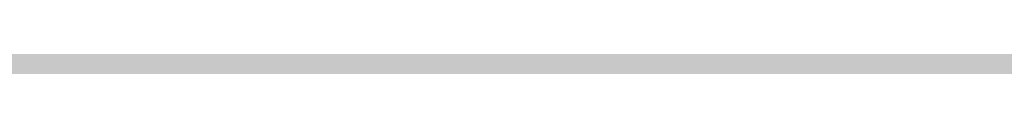
# Model space of a CAD drawing. Units: inches. Extents: x 2091 to 2899, y 967 to 2217.
# Tile 213 of 256: x 2203.2571 to 2203.4104, y 1152.2479 to 1152.2487. Entities that reach past the tile are written whole.
import ezdxf

# ---------------------------------------------------------------- set-up
doc = ezdxf.new("R2010")
doc.units = ezdxf.units.IN
doc.layers.add('A-WALL-PATT', color=141, linetype='Continuous', lineweight=13, true_color=0xadddf7)

msp = doc.modelspace()

# ---------------------------------------------------------------- hatches: boundary and pattern name
at = {"layer": 'A-WALL-PATT'}
h = msp.add_hatch(color=256, dxfattribs=at)
h.dxf.hatch_style = 1
h.paths.add_polyline_path([(2803.1436, 2050.91906), (2203.1436, 2050.91906), (2203.1436, 1090.91906), (2803.1436, 1090.91906)])
h.paths.add_polyline_path([(2635.79885, 1147.54046), (2674.52405, 1147.54046, 0.376086), (2678.52967, 1152.8802), (2678.52967, 1159.55647, 0.333335), (2674.52432, 1163.56185), (2674.52432, 1163.56185), (2674.52432, 1192.93439), (2635.80597, 1192.93439), (2597.08762, 1192.93439), (2597.08762, 1163.56185, 0.333335), (2593.08228, 1159.55647), (2593.08228, 1152.8802, 0.376086), (2597.08789, 1147.54046)], flags=0)
h.paths.add_polyline_path([(2436.01043, 1278.24078, 0.000483), (2435.95264, 1278.21503, -0.001328), (2435.93563, 1278.11169, -0.001711), (2436.11644, 1278.04076, 0.002185)], flags=0)
h.paths.add_polyline_path([(2794.1436, 1143.41906), (2794.1436, 1347.41906), (2543.37017, 1347.41906), (2543.37017, 1351.91906), (2794.1436, 1351.91906), (2794.1436, 1392.71355), (2793.9474, 1392.71355), (2793.9474, 1473.5369), (2794.1436, 1473.5369), (2794.1436, 1531.91906), (2650.1436, 1531.91906), (2650.1436, 1536.41906), (2794.1436, 1536.41906), (2794.1436, 1692.41906), (2609.37561, 1692.41906), (2609.37561, 1644.41906), (2604.87561, 1644.41906), (2604.87561, 1744.91906), (2609.37561, 1744.91906), (2609.37561, 1696.91906), (2794.1436, 1696.91906), (2794.1436, 1780.91906), (2609.6436, 1780.91906), (2493.87561, 1780.91906), (2493.87561, 1785.41906), (2609.6436, 1785.41906), (2794.1436, 1785.41906), (2794.1436, 1847.93882), (2793.95122, 1847.93882), (2793.95122, 1928.76217), (2794.1436, 1928.76217), (2794.1436, 1941.41906), (2614.1436, 1941.41906), (2614.1436, 1821.41906), (2609.6436, 1821.41906), (2609.6436, 1941.41906), (2392.1436, 1941.41906), (2392.1436, 1819.91906), (2387.6436, 1819.91906), (2387.6436, 1941.41906), (2212.1436, 1941.41906), (2212.1436, 1783.91906), (2392.1436, 1783.91906), (2392.1436, 1780.91906), (2212.1436, 1780.91906), (2212.1436, 1629.41906), (2387.6436, 1629.41906), (2387.6436, 1744.91906), (2392.1436, 1744.91906), (2392.1436, 1627.91906), (2317.1436, 1627.91906), (2317.1436, 1551.41906), (2317.1436, 1536.41906), (2459.38359, 1536.41906), (2459.38359, 1602.39648), (2463.88359, 1602.39648), (2463.88359, 1531.91906), (2456.6436, 1531.91906), (2456.6436, 1529.91906), (2452.1436, 1529.91906), (2452.1436, 1531.91906), (2312.6436, 1531.91906), (2312.6436, 1551.41906), (2306.1436, 1551.41906), (2306.1436, 1555.91906), (2308.1436, 1555.91906), (2308.1436, 1551.41906), (2312.6436, 1551.41906), (2312.6436, 1627.91906), (2212.1436, 1627.91906), (2212.1436, 1555.91906), (2270.1436, 1555.91906), (2270.1436, 1551.41906), (2212.1436, 1551.41906), (2212.1436, 1351.91906), (2272.1436, 1351.91906), (2272.1436, 1347.41906), (2212.1436, 1347.41906), (2212.1436, 1275.41906), (2308.1436, 1275.41906), (2308.1436, 1351.91906), (2452.1436, 1351.91906), (2452.1436, 1493.91906), (2456.6436, 1493.91906), (2456.6436, 1347.41906), (2312.6436, 1347.41906), (2312.6436, 1270.91906), (2212.1436, 1270.91906), (2212.1436, 1099.91906), (2281.23752, 1099.91906), (2282.87104, 1110.9138), (2282.00834, 1116.9966), (2278.55774, 1121.4204), (2268.20564, 1128.0562), (2272.08764, 1128.0562), (2273.81294, 1131.927), (2279.42034, 1134.6919), (2285.02784, 1135.2449), (2287.61584, 1137.4568), (2288.04714, 1138.0098), (2289.34114, 1140.7747), (2291.06654, 1139.6687), (2292.36054, 1135.2449), (2295.37984, 1136.9038), (2296.24254, 1135.7979), (2297.10524, 1133.033), (2300.12464, 1138.0098), (2303.14394, 1138.0098), (2304.43794, 1135.7979), (2303.14394, 1133.586), (2306.59464, 1134.6919), (2307.88874, 1133.033), (2310.90804, 1135.2449), (2313.92744, 1134.1389), (2315.62686, 1132.4271), (2308.32004, 1117.5496), (2290.20384, 1109.8079), (2288.90984, 1103.1721), (2289.27231, 1099.91906), (2434.91823, 1099.91906), (2431.59323, 1124.78806), (2429.93023, 1169.55306), (2430.92718, 1240.51969), (2435.65893, 1238.18613), (2437.13523, 1196.55406), (2438.79823, 1143.97306), (2442.67823, 1111.99806), (2446.55823, 1099.91906), (2794.1436, 1099.91906), (2794.1436, 1138.91906), (2548.03245, 1138.91906), (2548.03245, 1143.41906), (2548.03245, 1148.81906), (2546.66846, 1148.03156), (2528.68569, 1179.17862, 0.256256), (2512.03245, 1148.81906), (2512.03245, 1143.41906), (2512.03245, 1138.91906), (2507.53245, 1138.91906), (2507.53245, 1143.41906), (2507.53245, 1148.81906, 0.256256), (2490.8792, 1179.17862), (2472.89644, 1148.03156), (2471.53245, 1148.81906), (2471.53245, 1143.41906), (2467.03245, 1143.41906), (2467.03245, 1269.94579, 0.039061), (2460.90999, 1273.58006), (2467.03245, 1273.58006), (2467.03245, 1286.32536, 0.014511), (2465.21619, 1286.76191), (2467.03245, 1287.05258), (2467.03245, 1323.41906), (2471.53245, 1323.41906), (2471.53245, 1148.81906), (2489.53245, 1179.99597), (2490.89644, 1179.20847), (2490.8792, 1179.17862, -0.256256), (2507.53245, 1148.81906), (2507.53245, 1143.41906), (2512.03245, 1143.41906), (2512.03245, 1148.81906, -0.256256), (2528.68569, 1179.17862), (2528.66846, 1179.20847), (2530.03245, 1179.99597), (2548.03245, 1148.81906), (2548.03245, 1143.41906)], flags=16)
h.paths.add_polyline_path([(2607.76855, 1200.94508), (2607.76855, 1265.03063), (2597.08762, 1281.05201), (2619.78459, 1281.05201), (2627.79528, 1337.12686), (2635.79885, 1337.12686), (2643.81666, 1337.12686), (2651.82736, 1281.05201), (2674.52432, 1281.05201), (2663.8434, 1265.03063), (2663.8434, 1200.94508), (2635.80597, 1200.94508)], flags=0)
edge = h.paths.add_edge_path(flags=0)
edge.add_ellipse((13303.89622, 1272.99872), major_axis=(-10595.31304, 0), ratio=0.84230387009, start_angle=0.628237219, end_angle=0.6465541, ccw=False)
edge.add_ellipse((2711.70045, 1156.85268), major_axis=(2.21977, 0), ratio=0.8423039, start_angle=111.53524, end_angle=180.62824, ccw=False)
edge.add_ellipse((13303.15629, 1272.99872), major_axis=(-10593.02631, 0), ratio=0.84230386954, start_angle=0.528271472, end_angle=0.646554097, ccw=False)
edge.add_line((2710.7646, 1175.3333), (2710.12999, 1175.3333))
edge.add_ellipse((2710.12999, 1176.57978), major_axis=(1.47985, 0), ratio=0.8423039, start_angle=180, end_angle=270, ccw=False)
edge.add_line((2708.65014, 1176.57978), (2708.65014, 1200.78291))
edge.add_ellipse((2710.12999, 1200.78291), major_axis=(1.47985, 0), ratio=0.8423039, start_angle=90, end_angle=180, ccw=False)
edge.add_line((2710.12999, 1202.02939), (2710.46508, 1202.02939))
edge.add_ellipse((13303.15629, 1272.99872), major_axis=(-10593.02631, 0), ratio=0.84230386954, start_angle=-0.090229089, end_angle=0.383866779, ccw=False)
edge.add_ellipse((2710.12999, 1290.92703), major_axis=(-1.47985, 0), ratio=0.8423039, start_angle=0, end_angle=90, ccw=False)
edge.add_line((2708.65014, 1290.92703), (2708.65014, 1315.13017))
edge.add_ellipse((2710.12999, 1315.13017), major_axis=(-1.47985, 0), ratio=0.8423039, start_angle=-90, end_angle=0, ccw=False)
edge.add_line((2710.12999, 1316.37665), (2710.70631, 1316.37665))
edge.add_ellipse((3238.40172, 1296.28957), major_axis=(528.234, 0), ratio=0.84230387, start_angle=176.3495724, end_angle=177.8200497, ccw=False)
edge.add_ellipse((2775.06304, 1071.4507), major_axis=(313.30776, 0), ratio=0.84230387, start_angle=102.1259656, end_angle=103.780529, ccw=False)
edge.add_ellipse((2775.06304, 1078.3057), major_axis=(-305.30289, 0), ratio=0.84230387, start_angle=-79.790461, end_angle=-77.5553727, ccw=False)
edge.add_ellipse((2695.14177, 1541.97538), major_axis=(-250.96022, 0), ratio=0.84230387, start_angle=99.256566, end_angle=102.5549326)
edge.add_line((2741.41033, 1334.21426), (2747.13255, 1337.37848))
edge.add_ellipse((2747.53862, 1336.85748), major_axis=(-0.73992, 0), ratio=0.842304, start_angle=270, end_angle=307.93313, ccw=False)
edge.add_ellipse((2747.53862, 1336.85748), major_axis=(-0.73992, 0), ratio=0.842304, start_angle=232.06687, end_angle=270, ccw=False)
edge.add_line((2747.94469, 1337.37848), (2753.66691, 1334.21426))
edge.add_ellipse((2799.93547, 1541.97538), major_axis=(250.96022, 0), ratio=0.84230387, start_angle=257.4450674, end_angle=260.743434)
edge.add_ellipse((2720.01419, 1078.3057), major_axis=(305.30289, 0), ratio=0.84230387, start_angle=77.5553727, end_angle=79.790461, ccw=False)
edge.add_ellipse((2720.01419, 1071.4507), major_axis=(-313.30776, 0), ratio=0.84230387, start_angle=256.219471, end_angle=257.8740344, ccw=False)
edge.add_ellipse((2256.67551, 1296.28957), major_axis=(-528.234, 0), ratio=0.84230387, start_angle=182.1799503, end_angle=183.6504276, ccw=False)
edge.add_line((2784.37092, 1316.37665), (2784.94725, 1316.37665))
edge.add_ellipse((2784.94725, 1315.13017), major_axis=(1.47985, 0), ratio=0.8423039, start_angle=0, end_angle=90, ccw=False)
edge.add_line((2786.42709, 1315.13017), (2786.42709, 1290.92703))
edge.add_ellipse((2784.94725, 1290.92703), major_axis=(1.47985, 0), ratio=0.8423039, start_angle=270, end_angle=360, ccw=False)
edge.add_ellipse((-7808.07906, 1272.99872), major_axis=(10593.02631, 0), ratio=0.84230386954, start_angle=-0.383866779, end_angle=0.090229089, ccw=False)
edge.add_line((2784.61216, 1202.02939), (2784.94725, 1202.02939))
edge.add_ellipse((2784.94725, 1200.78291), major_axis=(1.47985, 0), ratio=0.8423039, start_angle=0, end_angle=90, ccw=False)
edge.add_line((2786.42709, 1200.78291), (2786.42709, 1176.57978))
edge.add_ellipse((2784.94725, 1176.57978), major_axis=(-1.47985, 0), ratio=0.8423039, start_angle=90, end_angle=180, ccw=False)
edge.add_line((2784.94725, 1175.3333), (2784.31264, 1175.3333))
edge.add_ellipse((-7808.07906, 1272.99872), major_axis=(10593.02631, 0), ratio=0.84230386954, start_angle=-0.618643196, end_angle=-0.528271472, ccw=False)
edge.add_ellipse((2783.37678, 1156.85268), major_axis=(-2.21977, 0), ratio=0.8423039, start_angle=179.37176, end_angle=248.46476, ccw=False)
edge.add_ellipse((-7808.81898, 1272.99872), major_axis=(-10595.31304, 0), ratio=0.84230386576, start_angle=179.353445923, end_angle=179.371762803, ccw=False)
edge.add_ellipse((2780.2973, 1153.50079), major_axis=(-5.24643, 0), ratio=0.8423039, start_angle=90, end_angle=179.35345, ccw=False)
edge.add_line((2780.2973, 1149.08171), (2714.77993, 1149.08171))
edge.add_ellipse((2714.77993, 1153.50079), major_axis=(5.24643, 0), ratio=0.8423039, start_angle=180.64655, end_angle=270, ccw=False)
edge = h.paths.add_edge_path(flags=0)
edge.add_line((2718.18737, 1151.00783), (2718.18737, 1170.47236))
edge.add_ellipse((2721.14706, 1170.47236), major_axis=(-2.95969, 0), ratio=0.8423039, start_angle=-90, end_angle=0, ccw=False)
edge.add_line((2721.14706, 1172.96532), (2773.93017, 1172.96532))
edge.add_ellipse((2773.93017, 1170.47236), major_axis=(-2.95969, 0), ratio=0.8423039, start_angle=180, end_angle=270, ccw=False)
edge.add_line((2776.88987, 1170.47236), (2776.88987, 1151.00783))
edge.add_line((2776.88987, 1151.00783), (2718.18737, 1151.00783))
edge = h.paths.add_edge_path(flags=0)
edge.add_line((2718.18737, 1180.23415), (2718.18737, 1199.05783))
edge.add_ellipse((2747.53862, 1320.39864), major_axis=(147.01792, 0), ratio=0.84230387, start_angle=256.4018653, end_angle=283.5981347)
edge.add_line((2776.88987, 1199.05783), (2776.88987, 1180.23415))
edge.add_ellipse((2747.53862, 1301.57496), major_axis=(147.01792, 0), ratio=0.84230387, start_angle=256.4018653, end_angle=283.5981347, ccw=False)
edge = h.paths.add_edge_path(flags=0)
edge.add_ellipse((13303.15629, 1272.99872), major_axis=(-10591.54646, 0), ratio=0.84230386955, start_angle=0.055594314, end_angle=0.377764194, ccw=False)
edge.add_line((2711.61686, 1262.72171), (2715.66741, 1249.4954))
edge.add_ellipse((6413.89196, 1241.69192), major_axis=(-3698.23616, 0), ratio=0.8423038695, start_angle=-0.12089737, end_angle=0.36407635)
edge.add_line((2715.76104, 1218.19245), (2711.93431, 1203.16736))
edge = h.paths.add_edge_path(flags=0)
edge.add_line((2718.18737, 1251.07457), (2716.00249, 1267.45044))
edge.add_ellipse((2742.15117, 1202.18954), major_axis=(81.77258, 0), ratio=0.84230387, start_angle=94.277421, end_angle=111.8349538, ccw=False)
edge.add_line((2737.00975, 1270.93063), (2758.06748, 1270.93063))
edge.add_ellipse((2752.92606, 1202.18954), major_axis=(81.77258, 0), ratio=0.84230387, start_angle=68.1650462, end_angle=85.722579, ccw=False)
edge.add_line((2779.07475, 1267.45044), (2776.88987, 1251.07457))
edge.add_ellipse((2750.33806, 1187.88536), major_axis=(79.57966, 0), ratio=0.84230387, start_angle=67.2080851, end_angle=85.1299304)
edge.add_line((2756.03466, 1254.74366), (2739.04258, 1254.74366))
edge.add_ellipse((2744.73917, 1187.88536), major_axis=(79.57966, 0), ratio=0.84230387, start_angle=94.8700696, end_angle=112.7919149)
edge = h.paths.add_edge_path(flags=0)
edge.add_line((2783.14293, 1203.16736), (2779.31619, 1218.19245))
edge.add_ellipse((-918.81473, 1241.69192), major_axis=(3698.23616, 0), ratio=0.8423038695, start_angle=-0.36407635, end_angle=0.12089737)
edge.add_line((2779.40983, 1249.4954), (2783.46037, 1262.72171))
edge.add_ellipse((-7808.07906, 1272.99872), major_axis=(-10591.54646, 0), ratio=0.84230386954, start_angle=179.622235806, end_angle=179.944405687, ccw=False)
edge = h.paths.add_edge_path(flags=0)
edge.add_ellipse((2734.20089, 1286.69044), major_axis=(-0.35661, 6.34008), ratio=0.6038336, start_angle=89.002014, end_angle=253.657408, ccw=False)
edge.add_line((2730.369, 1286.54181), (2730.369, 1301.35198))
edge.add_line((2730.369, 1301.35198), (2735.91331, 1305.2148))
edge.add_ellipse((2736.38492, 1304.73456), major_axis=(0.73992, 0), ratio=0.842304, start_angle=90, end_angle=134.48021, ccw=False)
edge.add_line((2736.38492, 1305.3578), (2738.03278, 1305.3578))
edge.add_line((2738.03278, 1305.3578), (2738.03278, 1307.70793))
edge.add_ellipse((2794.20164, 1307.70793), major_axis=(56.16886, 0), ratio=0.84230387, start_angle=150.56143, end_angle=180, ccw=False)
edge.add_ellipse((2700.87559, 1307.70793), major_axis=(-56.16886, 0), ratio=0.84230387, start_angle=180, end_angle=209.43857, ccw=False)
edge.add_line((2757.04445, 1307.70793), (2757.04445, 1305.3578))
edge.add_line((2757.04445, 1305.3578), (2758.69232, 1305.3578))
edge.add_ellipse((2758.69232, 1304.73456), major_axis=(-0.73992, 0), ratio=0.842304, start_angle=225.51979, end_angle=270, ccw=False)
edge.add_line((2759.16392, 1305.2148), (2764.70823, 1301.35198))
edge.add_line((2764.70823, 1301.35198), (2764.70823, 1286.54181))
edge.add_ellipse((2760.87634, 1286.69044), major_axis=(0.35661, 6.34008), ratio=0.6038336, start_angle=106.342592, end_angle=270.997986, ccw=False)
edge.add_line((2757.04445, 1285.79709), (2757.04445, 1307.70793))
edge.add_ellipse((2700.87559, 1307.70793), major_axis=(-56.16886, 0), ratio=0.84230387, start_angle=180, end_angle=209.43857)
edge.add_ellipse((2794.20164, 1307.70793), major_axis=(56.16886, 0), ratio=0.84230387, start_angle=150.56143, end_angle=180)
edge.add_line((2738.03278, 1307.70793), (2738.03278, 1285.79709))
h.paths.add_polyline_path([(2417.81227, 1104.4497), (2413.49227, 1102.5297), (2410.61227, 1103.9697), (2409.17227, 1106.3697), (2407.25227, 1107.3297), (2406.29227, 1109.7297), (2405.33227, 1114.0497), (2405.33227, 1117.8897), (2406.29227, 1120.1297), (2407.25227, 1119.8097), (2408.84832, 1118.32766), (2410.17395, 1119.42417), (2410.21127, 1120.4057), (2411.04073, 1121.41905), (2410.69927, 1119.8587), (2410.17395, 1119.42417), (2410.08845, 1117.17611), (2411.13284, 1116.20632), (2413.97227, 1119.3297), (2416.85227, 1120.7697), (2416.86972, 1120.79878), (2417.03507, 1119.40512), (2417.89621, 1118.14338), (2418.29227, 1118.3697), (2419.54445, 1120.03927), (2419.36092, 1118.38749), (2419.03211, 1119.35615), (2418.39894, 1118.51193), (2419.25227, 1114.5297), (2418.79409, 1107.19879)], flags=0)
h.paths.add_polyline_path([(2508.87017, 1347.41906), (2508.37017, 1347.41906), (2508.37017, 1351.91906), (2508.87017, 1351.91906)], flags=0)
h.paths.add_polyline_path([(2473.37017, 1347.41906), (2472.37017, 1347.41906), (2467.87017, 1347.41906), (2467.87017, 1455.41906), (2472.37017, 1455.41906), (2472.37017, 1352.41906), (2473.37017, 1352.41906)], flags=0)
h.paths.add_polyline_path([(2352.10624, 1217.4462), (2349.22624, 1218.8862), (2347.78624, 1221.2862), (2345.86624, 1222.2462), (2344.90624, 1224.6462), (2343.94624, 1228.9662), (2343.94624, 1232.8062), (2344.90624, 1235.0462), (2345.86624, 1234.7262), (2347.46229, 1233.24415), (2348.78792, 1234.34066), (2348.82524, 1235.3222), (2349.6547, 1236.33555), (2349.31324, 1234.7752), (2348.78792, 1234.34066), (2348.70242, 1232.0926), (2349.74681, 1231.12282), (2352.58624, 1234.2462), (2355.46624, 1235.6862), (2355.48369, 1235.71528), (2355.64904, 1234.32161), (2356.51018, 1233.05988), (2356.90624, 1233.2862), (2358.15842, 1234.95576), (2357.97489, 1233.30398), (2357.64608, 1234.27264), (2357.01291, 1233.42842), (2357.86624, 1229.4462), (2357.40806, 1222.11529), (2356.42624, 1219.3662)], flags=0)
h.paths.add_polyline_path([(2348.2968, 1112.22442), (2347.0138, 1112.31042), (2345.5298, 1114.12742), (2345.7318, 1115.85842), (2346.8118, 1116.98242), (2346.8118, 1114.64642), (2345.8668, 1114.21442), (2346.8798, 1114.30042)], flags=0)
h.paths.add_polyline_path([(2347.0138, 1110.92642), (2346.2718, 1110.49342), (2346.6098, 1111.18642)], flags=0)
h.paths.add_polyline_path([(2345.8668, 1118.19442), (2345.5298, 1117.32942), (2343.7078, 1118.02142), (2344.3828, 1118.62642)], flags=0)
h.paths.add_polyline_path([(2346.6768, 1109.28242), (2346.0698, 1108.07142), (2345.8668, 1110.06142)], flags=0)
h.paths.add_polyline_path([(2345.0568, 1119.75142), (2343.6398, 1119.75142), (2343.9778, 1121.13542)], flags=0)
h.paths.add_polyline_path([(2345.2598, 1116.55042), (2345.1248, 1115.85842), (2344.9218, 1115.68542), (2344.7198, 1116.37742)], flags=0)
h.paths.add_polyline_path([(2345.6648, 1112.31042), (2345.4618, 1111.53242), (2344.0448, 1111.96442), (2344.6518, 1112.57042)], flags=0)
h.paths.add_polyline_path([(2345.1918, 1113.34942), (2344.4498, 1113.86842), (2344.7198, 1114.38742)], flags=0)
h.paths.add_polyline_path([(2344.6518, 1116.80942), (2344.1798, 1115.68542), (2344.6518, 1115.33942), (2343.9098, 1114.90642), (2343.0328, 1115.94442), (2343.6398, 1116.46342)], flags=0)
h.paths.add_polyline_path([(2345.8668, 1106.68642), (2344.9898, 1105.56242), (2344.5168, 1106.60042)], flags=0)
h.paths.add_polyline_path([(2344.8548, 1110.06142), (2344.5168, 1109.28242), (2344.1128, 1109.71542)], flags=0)
h.paths.add_polyline_path([(2344.0448, 1113.52242), (2343.4378, 1113.08942), (2342.7628, 1113.95442)], flags=0)
h.paths.add_polyline_path([(2344.3148, 1111.01242), (2342.9648, 1110.32042), (2342.9648, 1111.09942)], flags=0)
h.paths.add_polyline_path([(2345.1248, 1104.69742), (2344.5848, 1103.74542), (2344.4498, 1104.26442)], flags=0)
h.paths.add_polyline_path([(2342.8298, 1121.22242), (2341.7498, 1120.53042), (2340.5358, 1121.04942), (2340.1308, 1121.82842), (2340.6708, 1122.95242), (2341.1428, 1121.82842), (2341.6148, 1122.00142)], flags=0)
h.paths.add_polyline_path([(2342.9648, 1119.75142), (2343.0328, 1118.45342), (2342.0878, 1118.02142), (2342.0198, 1119.49142)], flags=0)
h.paths.add_polyline_path([(2342.6948, 1116.89642), (2341.9528, 1116.63642), (2342.0198, 1117.32942)], flags=0)
h.paths.add_polyline_path([(2343.0328, 1112.22442), (2342.0198, 1111.79142), (2341.5478, 1112.22442), (2342.3578, 1113.34942)], flags=0)
h.paths.add_polyline_path([(2343.7748, 1104.43742), (2342.6278, 1102.88042), (2342.6948, 1104.61042), (2343.4378, 1105.12942)], flags=0)
h.paths.add_polyline_path([(2342.0198, 1115.07942), (2340.8058, 1115.51242), (2340.9408, 1116.37742)], flags=0)
h.paths.add_polyline_path([(2341.4808, 1120.09742), (2341.4808, 1119.40542), (2341.0758, 1119.57842), (2341.1428, 1120.09742)], flags=0)
h.paths.add_polyline_path([(2341.8178, 1114.47342), (2340.9408, 1113.08942), (2340.8058, 1114.56042)], flags=0)
h.paths.add_polyline_path([(2341.1428, 1118.54042), (2340.9408, 1116.98242), (2339.0508, 1117.67542), (2339.0508, 1118.62642)], flags=0)
h.paths.add_polyline_path([(2342.6948, 1101.66842), (2341.9528, 1101.84142), (2342.5598, 1102.36142)], flags=0)
h.paths.add_polyline_path([(2340.3328, 1119.66542), (2338.4438, 1119.57842), (2337.9038, 1120.35742), (2339.6578, 1120.61642)], flags=0)
h.paths.add_polyline_path([(2340.3328, 1115.33942), (2340.0628, 1113.69542), (2339.3878, 1115.33942)], flags=0)
h.paths.add_polyline_path([(2341.8178, 1103.83142), (2341.5478, 1102.88042), (2341.1428, 1103.65842)], flags=0)
h.paths.add_polyline_path([(2339.0508, 1122.86642), (2337.2958, 1121.82842), (2337.0938, 1123.12542), (2337.7688, 1123.81842)], flags=0)
h.paths.add_polyline_path([(2339.1178, 1121.74142), (2338.8478, 1121.22242), (2338.1738, 1121.04942), (2338.3758, 1121.56842)], flags=0)
h.paths.add_polyline_path([(2339.1858, 1119.31942), (2338.6458, 1118.71342), (2338.2408, 1118.10742), (2338.2408, 1118.88642)], flags=0)
h.paths.add_polyline_path([(2341.1428, 1101.92842), (2340.6028, 1101.23642), (2340.0628, 1101.84142), (2340.6028, 1102.36142)], flags=0)
h.paths.add_polyline_path([(2337.6338, 1117.76142), (2336.6208, 1118.28042), (2337.2958, 1118.97242)], flags=0)
h.paths.add_polyline_path([(2336.8238, 1119.57842), (2334.7988, 1118.97242), (2335.2038, 1120.35742), (2336.5538, 1120.87642)], flags=0)
h.paths.add_polyline_path([(2339.1178, 1100.45742), (2337.3638, 1100.54342), (2336.7558, 1101.23642)], flags=0)
h.paths.add_polyline_path([(2336.3508, 1122.43342), (2336.0138, 1121.91442), (2334.9338, 1122.43342), (2334.5288, 1123.47142), (2335.7438, 1122.77942)], flags=0)
h.paths.add_polyline_path([(2334.7318, 1120.87642), (2334.2588, 1120.35742), (2334.0568, 1120.78942), (2334.5968, 1121.30842)], flags=0)
h.paths.add_polyline_path([(2334.4618, 1122.17442), (2332.5718, 1121.30842), (2331.3568, 1122.17442), (2332.0998, 1122.86642)], flags=0)
h.paths.add_polyline_path([(2334.2588, 1118.54042), (2333.3818, 1118.45342), (2333.6518, 1119.31942)], flags=0)
h.paths.add_polyline_path([(2335.5418, 1102.27442), (2334.1918, 1102.62042), (2335.2718, 1103.31242)], flags=0)
h.paths.add_polyline_path([(2332.7068, 1119.66542), (2331.6948, 1120.44342), (2332.5048, 1120.78942)], flags=0)
h.paths.add_polyline_path([(2334.7318, 1101.14942), (2333.5168, 1101.58242), (2333.9888, 1101.75542)], flags=0)
h.paths.add_polyline_path([(2332.6398, 1116.63642), (2331.0868, 1116.29042), (2331.9648, 1118.19442)], flags=0)
h.paths.add_polyline_path([(2330.7498, 1121.56842), (2330.2768, 1120.27042), (2328.5228, 1119.31942), (2328.9948, 1121.04942)], flags=0)
h.paths.add_polyline_path([(2330.7498, 1118.62642), (2330.0078, 1117.50242), (2329.8728, 1118.02142)], flags=0)
h.paths.add_polyline_path([(2332.0998, 1102.36142), (2330.5468, 1102.01442), (2331.6948, 1102.96642)], flags=0)
h.paths.add_polyline_path([(2329.5348, 1113.60842), (2329.0628, 1112.31042), (2328.5898, 1113.34942)], flags=0)
h.paths.add_polyline_path([(2328.3878, 1117.84842), (2327.5098, 1116.55042), (2327.1728, 1117.76142)], flags=0)
h.paths.add_polyline_path([(2329.7378, 1106.51342), (2329.5348, 1105.30242), (2328.2528, 1106.08142)], flags=0)
h.paths.add_polyline_path([(2328.6578, 1114.38742), (2328.0498, 1114.12742), (2328.3198, 1114.90642)], flags=0)
h.paths.add_polyline_path([(2328.3198, 1112.22442), (2327.1058, 1112.13742), (2326.7008, 1112.65642)], flags=0)
h.paths.add_polyline_path([(2326.9028, 1115.25242), (2326.7008, 1114.12742), (2325.2158, 1113.60842), (2326.0928, 1115.33942)], flags=0)
h.paths.add_polyline_path([(2326.6328, 1108.33042), (2326.0928, 1107.37942), (2325.8908, 1108.50342), (2326.4978, 1109.10942)], flags=0)
h.paths.add_polyline_path([(2615.1436, 1531.91906), (2609.6436, 1531.91906), (2609.6436, 1620.41906), (2614.1436, 1620.41906), (2614.1436, 1536.41906), (2615.1436, 1536.41906)], flags=0)
h.paths.add_polyline_path([(2545.1436, 1563.41906), (2464.1436, 1563.41906), (2464.1436, 1632.41906), (2509.1436, 1632.41906), (2509.1436, 1627.91906), (2509.1436, 1603.91906), (2468.6436, 1603.91906), (2468.6436, 1567.91906), (2540.6436, 1567.91906), (2540.6436, 1591.91906), (2545.1436, 1591.91906)], flags=0)
h.paths.add_polyline_path([(2388.96905, 1549.98573), (2357.43418, 1549.98573), (2357.43418, 1623.36078), (2399.36278, 1623.36078), (2435.68947, 1623.36078), (2435.59255, 1602.55927), (2435.59255, 1602.39648), (2388.96905, 1602.39648)], flags=0)
h.paths.add_polyline_path([(2388.88063, 1555.80915), (2374.90443, 1555.80915), (2374.90443, 1600.57156), (2374.90443, 1615.45765), (2406.35088, 1615.45765), (2406.35088, 1618.93943), (2412.17429, 1615.45765), (2406.35088, 1611.97586), (2406.35088, 1615.45765), (2388.88063, 1615.45765)], flags=0)
h.paths.add_polyline_path([(2568.87561, 1644.41906), (2453.37561, 1644.41906), (2453.37561, 1785.41906), (2457.87561, 1785.41906), (2457.87561, 1648.91906), (2568.87561, 1648.91906)], flags=0)
h.paths.add_polyline_path([(2212.1436, 1945.91906), (2212.1436, 2041.91906), (2794.1436, 2041.91906), (2794.1436, 1945.91906)], flags=16)
h.paths.add_polyline_path([(2271.08273, 1964.31724), (2776.85297, 1964.31724), (2776.85297, 2037.16962), (2271.08273, 2037.16962)], flags=8)
h.paths.add_polyline_path([(2380.64929, 1536.82414), (2461.04081, 1536.82414), (2461.04081, 1554.65259), (2380.64929, 1554.65259)], flags=8)
h.paths.add_polyline_path([(2240.75571, 1609.72545), (2309.18583, 1609.72545), (2309.18583, 1617.6982), (2240.75571, 1617.6982)], flags=8)
h.paths.add_polyline_path([(2212.67726, 1313.5041), (2282.59152, 1313.5041), (2282.59152, 1322.74524), (2212.67726, 1322.74524)], flags=8)
h.paths.add_polyline_path([(2457.11198, 1114.77857), (2558.48158, 1114.77857), (2558.48158, 1142.21968), (2457.11198, 1142.21968)], flags=8)
h.paths.add_polyline_path([(2473.44234, 1273.01007), (2604.64123, 1273.01007), (2604.64123, 1318.34693), (2473.44234, 1318.34693)], flags=8)
h.paths.add_polyline_path([(2638.8763, 1626.97743), (2684.25037, 1627.97674), (2684.03848, 1637.59749), (2638.66442, 1636.59819)], flags=8)
h.paths.add_polyline_path([(2537.59055, 1453.79345), (2628.38955, 1453.79345), (2628.38955, 1475.34481), (2537.59055, 1475.34481)], flags=8)
h.paths.add_polyline_path([(2504.13764, 1714.6324), (2554.64719, 1714.6324), (2554.64719, 1730.23771), (2504.13764, 1730.23771)], flags=8)
h.paths.add_polyline_path([(2487.50118, 1575.65187), (2535.09712, 1575.65187), (2535.09712, 1598.37765), (2487.50118, 1598.37765)], flags=8)
h.paths.add_polyline_path([(2709.0994, 1735.71028), (2740.0166, 1735.71028), (2740.0166, 1749.93764), (2709.0994, 1749.93764)], flags=8)
h.paths.add_polyline_path([(2442.43842, 1792.17166), (2564.72884, 1792.17166), (2564.72884, 1842.00016), (2442.43842, 1842.00016)], flags=8)
h.paths.add_polyline_path([(2655.8158, 1809.64408), (2789.52014, 1806.6938), (2790.08498, 1832.29164), (2656.38064, 1835.24192)], flags=8)
h.paths.add_polyline_path([(2234.8427, 1797.72014), (2368.59285, 1794.76885), (2369.16072, 1820.50413), (2235.41056, 1823.45542)], flags=8)
h.paths.add_polyline_path([(2245.13847, 1644.00633), (2398.42773, 1640.6239), (2398.99484, 1666.32482), (2245.70557, 1669.70725)], flags=8)
h.paths.add_polyline_path([(2306.14285, 1431.16852), (2413.76831, 1428.79369), (2414.33315, 1454.39153), (2306.70768, 1456.76636)], flags=8)
h.paths.add_polyline_path([(2306.83458, 1458.23314), (2393.38048, 1456.32345), (2393.93281, 1481.35436), (2307.38691, 1483.26405)], flags=8)

doc.saveas('drawing.dxf')
